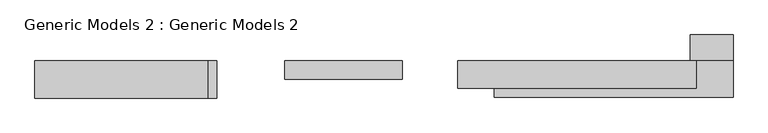
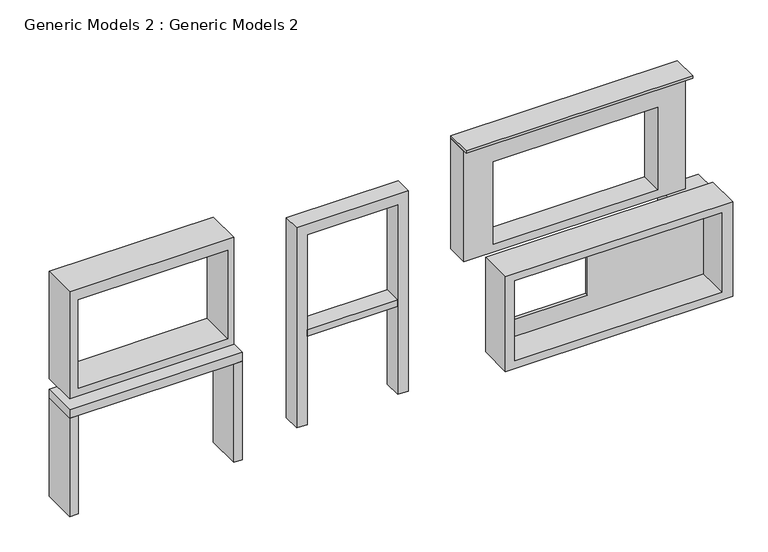
"""IFC4 building model written with IfcOpenShell, lengths in millimetres: proxy geometry, Generic Models 2 : Generic Models 2."""

from ifc_helpers import new_model, si_unit, frame, origin, origin_with_axes, place, context, project, spatial, polyline, outline, extrude, source, transform, mapped, element, save


def generic_models_2_generic_models_2_1d31d6de(model_context):
    return source(origin(), model_context, "Body", "SweptSolid", [
        extrude(outline(polyline([(13897.5944752, -14083.6014605), (7801.5944752, -14083.6014605), (7801.5944752, -13376.4602599), (13897.5944752, -13376.4602599), (13897.5944752, -14083.6014605)])), frame((0.0, 0.0, 6400.8), z_axis=(0.0, 0.0, 1.0), x_axis=(1.0, 0.0, 0.0)), (0.0, 0.0, 1.0), 76.2),
        extrude(outline(polyline([(6400.8, 13753.439189), (6400.8, 7801.5944752), (3253.5878782, 7801.5944752), (3253.5878782, 13753.439189), (6400.8, 13753.439189)]), holes=[polyline([(5829.0338442, 13012.9903499), (3479.8, 13012.9903499), (3479.8, 8593.3903499), (5829.0338442, 8593.3903499), (5829.0338442, 13012.9903499)])]), frame((0.0, -13986.0602599, 0.0), z_axis=(0.0, 1.0, 0.0), x_axis=(0.0, 0.0, 1.0)), (0.0, 0.0, 1.0), 609.6),
        extrude(outline(polyline([(2692.731124, 14845.639189), (2692.731124, 8734.9360339), (0.0, 8734.9360339), (0.0, 14845.639189), (2692.731124, 14845.639189)]), holes=[polyline([(225.6756618, 14553.539189), (225.6756618, 8990.939189), (2489.531124, 8990.939189), (2489.531124, 14553.539189), (225.6756618, 14553.539189)])]), frame((0.0, -14303.3338598, 0.0), z_axis=(0.0, 1.0, 0.0), x_axis=(0.0, 0.0, 1.0)), (0.0, 0.0, 1.0), 926.8735998),
        extrude(outline(polyline([(225.6756618, 14615.8010584), (2489.531124, 14615.8010584), (2489.531124, 11429.339189), (718.1429127, 11429.339189), (718.1429127, 8990.939189), (225.6756618, 8990.939189), (225.6756618, 14615.8010584)])), frame((0.0, -13452.6602599, 0.0), z_axis=(0.0, 1.0, 0.0), x_axis=(0.0, 0.0, 1.0)), (0.0, 0.0, 1.0), 76.2),
        extrude(outline(polyline([(14845.5874203, -13376.4602599), (13753.439189, -13376.4602599), (13753.439189, -12714.9746756), (14845.5874203, -12714.9746756), (14845.5874203, -13376.4602599)])), origin_with_axes(), (0.0, 0.0, 1.0), 2511.7877969),
        extrude(outline(polyline([(6095.339189, -13852.2176249), (3656.939189, -13852.2176249), (3656.939189, -13376.4602599), (6095.339189, -13376.4602599), (6095.339189, -13852.2176249)])), frame((0.0, 0.0, 2511.7877969), z_axis=(0.0, 0.0, 1.0), x_axis=(1.0, 0.0, 0.0)), (0.0, 0.0, 1.0), 184.8454523),
        extrude(outline(polyline([(0.0, 3377.539189), (0.0, 3656.939189), (5393.2664984, 3656.939189), (5393.2664984, 6095.339189), (0.0, 6095.339189), (0.0, 6378.8273334), (5692.5645868, 6378.8273334), (5692.5645868, 3377.539189), (0.0, 3377.539189)])), frame((0.0, -13852.2176249, 0.0), z_axis=(0.0, 1.0, 0.0), x_axis=(0.0, 0.0, 1.0)), (0.0, 0.0, 1.0), 475.757365),
        extrude(outline(polyline([(6400.8, 1409.039189), (6400.8, -3010.560811), (3352.8, -3010.560811), (3352.8, 1409.039189), (6400.8, 1409.039189)]), holes=[polyline([(6096.0, -2781.960811), (6096.0, 1244.917851), (3573.1395696, 1244.917851), (3573.1395696, -2781.960811), (6096.0, -2781.960811)])]), frame((0.0, -14328.5451307, 0.0), z_axis=(0.0, 1.0, 0.0), x_axis=(0.0, 0.0, 1.0)), (0.0, 0.0, 1.0), 952.0848708),
        extrude(outline(polyline([(1637.639189, -14328.5451307), (-3010.560811, -14328.5451307), (-3010.560811, -13376.4602599), (1637.639189, -13376.4602599), (1637.639189, -14328.5451307)])), frame((0.0, 0.0, 2801.7973469), z_axis=(0.0, 0.0, 1.0), x_axis=(1.0, 0.0, 0.0)), (0.0, 0.0, 1.0), 246.2026531),
        extrude(outline(polyline([(1637.639189, -13376.4602599), (1637.639189, -14328.5451307), (1409.039189, -14328.5451307), (1409.039189, -13376.4602599), (1637.639189, -13376.4602599)])), origin_with_axes(), (0.0, 0.0, 1.0), 2801.7973469),
        extrude(outline(polyline([(-3010.560811, -14328.5451307), (-3010.560811, -13376.4602599), (-2781.960811, -13376.4602599), (-2781.960811, -14328.5451307), (-3010.560811, -14328.5451307)])), origin_with_axes(), (0.0, 0.0, 1.0), 2801.7973469),
    ])


if __name__ == "__main__":
    model = new_model("IFC4")
    model_context = context("Model", 3, world=origin())
    ifc_project = project(units=[si_unit("LENGTHUNIT", "METRE", prefix="MILLI")], contexts=[model_context])
    site = spatial("IfcSite", under=ifc_project)
    building = spatial("IfcBuilding", under=site)
    placement = place(None, origin())
    generic_models_2_generic_models_2_shape = generic_models_2_generic_models_2_1d31d6de(model_context)
    element("IfcBuildingElementProxy", 1, Name="Generic Models 2 : Generic Models 2", ObjectType="Generic Models 2 : Generic Models 2", at=placement, inside=building, context=model_context, shape_type="MappedRepresentation", body=[
        mapped(generic_models_2_generic_models_2_shape, transform((0.0, 0.0, 0.0), x_axis=(1.0, 0.0, 0.0), y_axis=(0.0, 1.0, 0.0), z_axis=(0.0, 0.0, 1.0))),
    ])
    save(model, "model.ifc")
